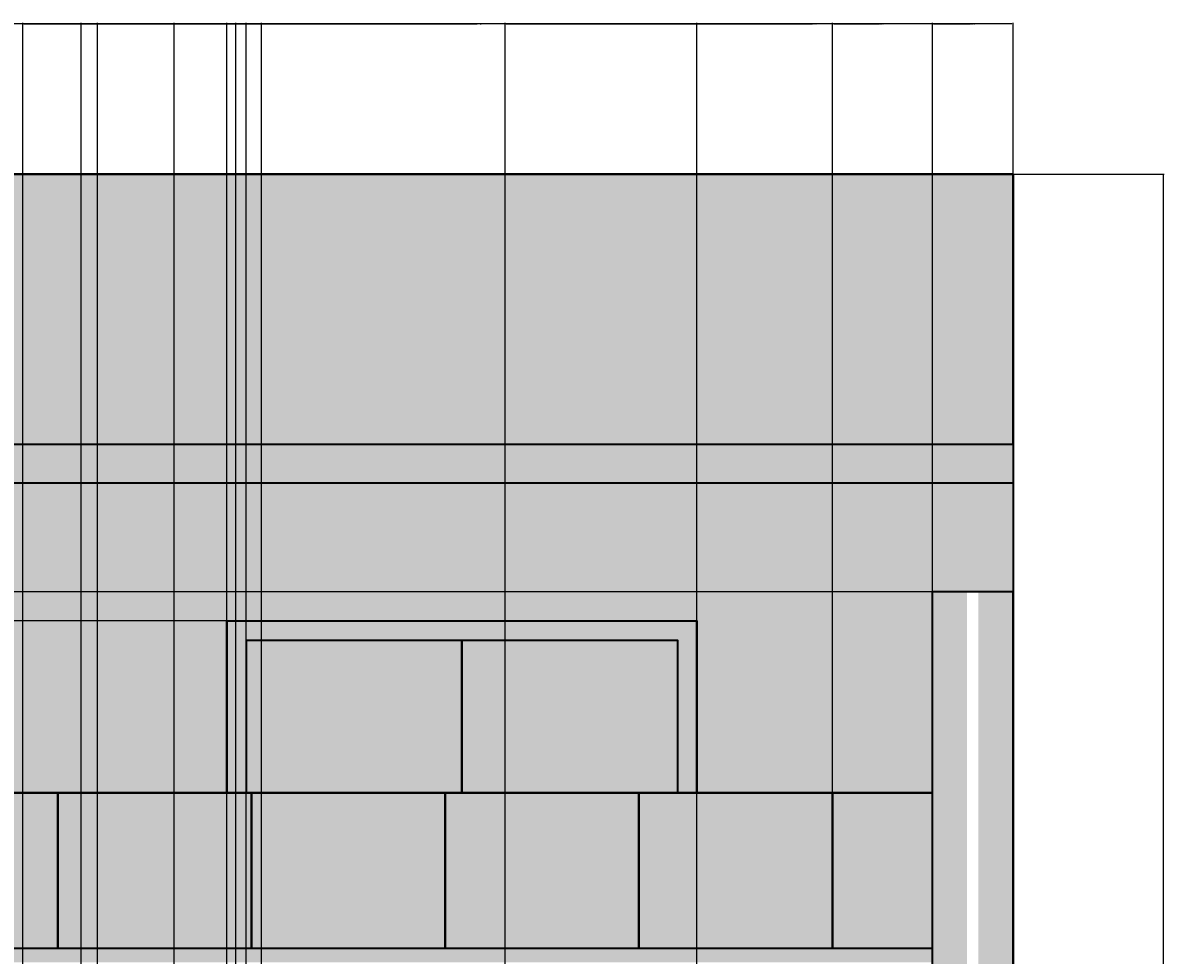
# Model space of a CAD drawing. Units: feet. Extents: x 2368 to 2738, y 1285 to 1782.
# Tile 6 of 6: x 2561 to 2738, y 1638 to 1782. Entities that reach past the tile are written whole.
import ezdxf

# ---------------------------------------------------------------- set-up
doc = ezdxf.new("R2010")
doc.units = ezdxf.units.FT
for name, color, linetype, lineweight in [('A-ANNO-DIMS', 2, 'Continuous', 18), ('A-ELEV', 7, 'Continuous', 35), ('A-ELEV-PATT', 252, 'Continuous', 13), ('A-GLAZ', 4, 'Continuous', 25)]:
    doc.layers.add(name, color=color, linetype=linetype, lineweight=lineweight)
doc.styles.get("Standard").update_dxf_attribs({"font": 'arial.ttf'})
doc.dimstyles.get("Standard").update_dxf_attribs({"dimtxt": 0.18, "dimasz": 0.18, "dimexe": 0.18, "dimexo": 0.0625, "dimgap": 0.09, "dimtad": 0, "dimtih": 1, "dimtoh": 1, "dimdec": 1, "dimzin": 0, "dimdsep": 46, "dimlunit": 3, "dimtxsty": 'Standard', "dimcen": 0.09, "dimadec": 0, "dimazin": 0, "dimtfac": 1, "dimtdec": 1, "dimtofl": 0, "dimtmove": 0, "dimatfit": 3, "dimfxl": 1, "dimtolj": 1, "dimtzin": 0, "dimarcsym": 0})

# ---------------------------------------------------------------- blocks, each defined once
blk = doc.blocks.new('*D1')
at = {"layer": 'A-ANNO-DIMS', "color": 0, "lineweight": -2, "transparency": 16777216}
for p, q in [((2391.54, 1662.92), (2391.54, 1782.11)), ((2391.72, 1781.93), (2552.46, 1781.93)), ((2713.98, 1781.93), (2553.25, 1781.93)), ((2714.16, 1758.74), (2714.16, 1782.11))]:
    blk.add_line(p, q, dxfattribs=at)
at = {"layer": 'A-ANNO-DIMS', "color": 0, "transparency": 16777216}
for points in [[(2391.72, 1781.96), (2391.72, 1781.9), (2391.54, 1781.93)], [(2713.98, 1781.96), (2713.98, 1781.9), (2714.16, 1781.93)]]:
    blk.add_solid(points, dxfattribs=at)
at = {"layer": 'Defpoints', "color": 0, "transparency": 16777216}
for p in [(2714.16, 1781.93), (2714.16, 1758.68), (2391.54, 1662.86)]:
    blk.add_point(p, dxfattribs=at)
at = {"layer": 'A-ANNO-DIMS', "color": 0, "transparency": 16777216, "insert": (2552.85, 1781.93), "char_height": 0.18, "attachment_point": 5}
blk.add_mtext('\\A1;322.6', dxfattribs=at)
blk = doc.blocks.new('*D2')
at = {"layer": 'A-ANNO-DIMS', "color": 0, "lineweight": -2, "transparency": 16777216}
for p, q in [((2714.23, 1758.68), (2737.59, 1758.68)), ((2737.41, 1758.5), (2737.41, 1533.95)), ((2737.41, 1309.04), (2737.41, 1533.58)), ((2714.23, 1308.86), (2737.59, 1308.86))]:
    blk.add_line(p, q, dxfattribs=at)
at = {"layer": 'A-ANNO-DIMS', "color": 0, "transparency": 16777216}
for points in [[(2737.38, 1758.5), (2737.44, 1758.5), (2737.41, 1758.68)], [(2737.38, 1309.04), (2737.44, 1309.04), (2737.41, 1308.86)]]:
    blk.add_solid(points, dxfattribs=at)
at = {"layer": 'Defpoints', "color": 0, "transparency": 16777216}
for p in [(2714.16, 1758.68), (2737.41, 1758.68), (2714.16, 1308.86)]:
    blk.add_point(p, dxfattribs=at)
at = {"layer": 'A-ANNO-DIMS', "color": 0, "transparency": 16777216, "insert": (2737.41, 1533.77), "char_height": 0.18, "attachment_point": 5}
blk.add_mtext('\\A1;449.8', dxfattribs=at)
blk = doc.blocks.new('*D33')
at = {"layer": 'A-ANNO-DIMS', "color": 0, "lineweight": -2, "transparency": 16777216}
for p, q in [((2592.41, 1461.2), (2592.41, 1782.11)), ((2592.59, 1781.93), (2593.76, 1781.93)), ((2595.23, 1781.93), (2594.06, 1781.93)), ((2595.41, 1458.2), (2595.41, 1782.11))]:
    blk.add_line(p, q, dxfattribs=at)
at = {"layer": 'A-ANNO-DIMS', "color": 0, "transparency": 16777216}
for points in [[(2592.59, 1781.96), (2592.59, 1781.9), (2592.41, 1781.93)], [(2595.23, 1781.96), (2595.23, 1781.9), (2595.41, 1781.93)]]:
    blk.add_solid(points, dxfattribs=at)
at = {"layer": 'Defpoints', "color": 0, "transparency": 16777216}
for p in [(2595.41, 1781.93), (2592.41, 1461.14), (2595.41, 1458.14)]:
    blk.add_point(p, dxfattribs=at)
at = {"layer": 'A-ANNO-DIMS', "color": 0, "transparency": 16777216, "insert": (2593.91, 1781.93), "char_height": 0.18, "attachment_point": 5}
blk.add_mtext('\\A1;3', dxfattribs=at)
blk = doc.blocks.new('*D34')
at = {"layer": 'A-ANNO-DIMS', "color": 0, "lineweight": -2, "transparency": 16777216}
for p, q in [((2560.8, 1466.16), (2560.8, 1782.11)), ((2560.98, 1781.93), (2597.75, 1781.93)), ((2635.31, 1781.93), (2598.54, 1781.93)), ((2635.49, 1466.16), (2635.49, 1782.11))]:
    blk.add_line(p, q, dxfattribs=at)
at = {"layer": 'A-ANNO-DIMS', "color": 0, "transparency": 16777216}
for points in [[(2560.98, 1781.96), (2560.98, 1781.9), (2560.8, 1781.93)], [(2635.31, 1781.96), (2635.31, 1781.9), (2635.49, 1781.93)]]:
    blk.add_solid(points, dxfattribs=at)
at = {"layer": 'Defpoints', "color": 0, "transparency": 16777216}
for p in [(2635.49, 1781.93), (2560.8, 1466.1), (2635.49, 1466.1)]:
    blk.add_point(p, dxfattribs=at)
at = {"layer": 'A-ANNO-DIMS', "color": 0, "transparency": 16777216, "insert": (2598.14, 1781.93), "char_height": 0.18, "attachment_point": 5}
blk.add_mtext('\\A1;74.69', dxfattribs=at)
blk = doc.blocks.new('*D35')
at = {"layer": 'A-ANNO-DIMS', "color": 0, "lineweight": -2, "transparency": 16777216}
for p, q in [((2635.49, 1466.16), (2635.49, 1782.11)), ((2635.67, 1781.93), (2668.18, 1781.93)), ((2701.48, 1781.93), (2668.97, 1781.93)), ((2701.66, 1466.16), (2701.66, 1782.11))]:
    blk.add_line(p, q, dxfattribs=at)
at = {"layer": 'A-ANNO-DIMS', "color": 0, "transparency": 16777216}
for points in [[(2635.67, 1781.96), (2635.67, 1781.9), (2635.49, 1781.93)], [(2701.48, 1781.96), (2701.48, 1781.9), (2701.66, 1781.93)]]:
    blk.add_solid(points, dxfattribs=at)
at = {"layer": 'Defpoints', "color": 0, "transparency": 16777216}
for p in [(2701.66, 1781.93), (2635.49, 1466.1), (2701.66, 1466.1)]:
    blk.add_point(p, dxfattribs=at)
at = {"layer": 'A-ANNO-DIMS', "color": 0, "transparency": 16777216, "insert": (2668.57, 1781.93), "char_height": 0.18, "attachment_point": 5}
blk.add_mtext('\\A1;66.17', dxfattribs=at)
blk = doc.blocks.new('*D39')
at = {"layer": 'A-ANNO-DIMS', "color": 0, "lineweight": -2, "transparency": 16777216}
for p, q in [((2701.6, 1662.86), (2368.11, 1662.86)), ((2368.29, 1662.68), (2368.29, 1651.02)), ((2368.29, 1638.99), (2368.29, 1650.65)), ((2701.6, 1638.81), (2368.11, 1638.81))]:
    blk.add_line(p, q, dxfattribs=at)
at = {"layer": 'A-ANNO-DIMS', "color": 0, "transparency": 16777216}
for points in [[(2368.26, 1662.68), (2368.32, 1662.68), (2368.29, 1662.86)], [(2368.26, 1638.99), (2368.32, 1638.99), (2368.29, 1638.81)]]:
    blk.add_solid(points, dxfattribs=at)
at = {"layer": 'Defpoints', "color": 0, "transparency": 16777216}
for p in [(2368.29, 1662.86), (2701.66, 1662.86), (2701.66, 1638.81)]:
    blk.add_point(p, dxfattribs=at)
at = {"layer": 'A-ANNO-DIMS', "color": 0, "transparency": 16777216, "insert": (2368.29, 1650.83), "char_height": 0.18, "attachment_point": 5}
blk.add_mtext('\\A1;24.042', dxfattribs=at)
blk = doc.blocks.new('*D40')
at = {"layer": 'A-ANNO-DIMS', "color": 0, "lineweight": -2, "transparency": 16777216}
for p, q in [((2701.6, 1693.98), (2368.11, 1693.98)), ((2368.29, 1693.8), (2368.29, 1678.6)), ((2368.29, 1663.04), (2368.29, 1678.24)), ((2701.6, 1662.86), (2368.11, 1662.86))]:
    blk.add_line(p, q, dxfattribs=at)
at = {"layer": 'A-ANNO-DIMS', "color": 0, "transparency": 16777216}
for points in [[(2368.26, 1693.8), (2368.32, 1693.8), (2368.29, 1693.98)], [(2368.26, 1663.04), (2368.32, 1663.04), (2368.29, 1662.86)]]:
    blk.add_solid(points, dxfattribs=at)
at = {"layer": 'Defpoints', "color": 0, "transparency": 16777216}
for p in [(2368.29, 1693.98), (2701.66, 1693.98), (2701.66, 1662.86)]:
    blk.add_point(p, dxfattribs=at)
at = {"layer": 'A-ANNO-DIMS', "color": 0, "transparency": 16777216, "insert": (2368.29, 1678.42), "char_height": 0.18, "attachment_point": 5}
blk.add_mtext('\\A1;31.13', dxfattribs=at)
blk = doc.blocks.new('*D54')
at = {"layer": 'A-ANNO-DIMS', "color": 0, "lineweight": -2, "transparency": 16777216}
for p, q in [((2560.78, 1609.97), (2560.78, 1782.11)), ((2560.96, 1781.93), (2564.98, 1781.93)), ((2569.66, 1781.93), (2565.63, 1781.93)), ((2569.84, 1609.97), (2569.84, 1782.11))]:
    blk.add_line(p, q, dxfattribs=at)
at = {"layer": 'A-ANNO-DIMS', "color": 0, "transparency": 16777216}
for points in [[(2560.96, 1781.96), (2560.96, 1781.9), (2560.78, 1781.93)], [(2569.66, 1781.96), (2569.66, 1781.9), (2569.84, 1781.93)]]:
    blk.add_solid(points, dxfattribs=at)
at = {"layer": 'Defpoints', "color": 0, "transparency": 16777216}
for p in [(2569.84, 1781.93), (2560.78, 1609.91), (2569.84, 1609.91)]:
    blk.add_point(p, dxfattribs=at)
at = {"layer": 'A-ANNO-DIMS', "color": 0, "transparency": 16777216, "insert": (2565.31, 1781.93), "char_height": 0.18, "attachment_point": 5}
blk.add_mtext('\\A1;9.06', dxfattribs=at)
blk = doc.blocks.new('*D55')
at = {"layer": 'A-ANNO-DIMS', "color": 0, "lineweight": -2, "transparency": 16777216}
for p, q in [((2569.84, 1609.97), (2569.84, 1782.11)), ((2570.02, 1781.93), (2576.72, 1781.93)), ((2584.06, 1781.93), (2577.35, 1781.93)), ((2584.24, 1609.97), (2584.24, 1782.11))]:
    blk.add_line(p, q, dxfattribs=at)
at = {"layer": 'A-ANNO-DIMS', "color": 0, "transparency": 16777216}
for points in [[(2570.02, 1781.96), (2570.02, 1781.9), (2569.84, 1781.93)], [(2584.06, 1781.96), (2584.06, 1781.9), (2584.24, 1781.93)]]:
    blk.add_solid(points, dxfattribs=at)
at = {"layer": 'Defpoints', "color": 0, "transparency": 16777216}
for p in [(2584.24, 1781.93), (2569.84, 1609.91), (2584.24, 1609.91)]:
    blk.add_point(p, dxfattribs=at)
at = {"layer": 'A-ANNO-DIMS', "color": 0, "transparency": 16777216, "insert": (2577.04, 1781.93), "char_height": 0.18, "attachment_point": 5}
blk.add_mtext('\\A1;14.4', dxfattribs=at)
blk = doc.blocks.new('*D56')
at = {"layer": 'A-ANNO-DIMS', "color": 0, "lineweight": -2, "transparency": 16777216}
for p, q in [((2593.78, 1609.97), (2593.78, 1782.11)), ((2593.96, 1781.93), (2595.62, 1781.93)), ((2597.6, 1781.93), (2595.93, 1781.93)), ((2597.78, 1609.97), (2597.78, 1782.11))]:
    blk.add_line(p, q, dxfattribs=at)
at = {"layer": 'A-ANNO-DIMS', "color": 0, "transparency": 16777216}
for points in [[(2593.96, 1781.96), (2593.96, 1781.9), (2593.78, 1781.93)], [(2597.6, 1781.96), (2597.6, 1781.9), (2597.78, 1781.93)]]:
    blk.add_solid(points, dxfattribs=at)
at = {"layer": 'Defpoints', "color": 0, "transparency": 16777216}
for p in [(2597.78, 1781.93), (2593.78, 1609.91), (2597.78, 1609.91)]:
    blk.add_point(p, dxfattribs=at)
at = {"layer": 'A-ANNO-DIMS', "color": 0, "transparency": 16777216, "insert": (2595.78, 1781.93), "char_height": 0.18, "attachment_point": 5}
blk.add_mtext('\\A1;4', dxfattribs=at)
blk = doc.blocks.new('*D57')
at = {"layer": 'A-ANNO-DIMS', "color": 0, "lineweight": -2, "transparency": 16777216}
for p, q in [((2569.84, 1609.97), (2569.84, 1782.11)), ((2570.02, 1781.93), (2570.71, 1781.93)), ((2572.19, 1781.93), (2571.5, 1781.93)), ((2572.37, 1609.97), (2572.37, 1782.11))]:
    blk.add_line(p, q, dxfattribs=at)
at = {"layer": 'A-ANNO-DIMS', "color": 0, "transparency": 16777216}
for points in [[(2570.02, 1781.96), (2570.02, 1781.9), (2569.84, 1781.93)], [(2572.19, 1781.96), (2572.19, 1781.9), (2572.37, 1781.93)]]:
    blk.add_solid(points, dxfattribs=at)
at = {"layer": 'Defpoints', "color": 0, "transparency": 16777216}
for p in [(2572.37, 1781.93), (2569.84, 1609.91), (2572.37, 1609.91)]:
    blk.add_point(p, dxfattribs=at)
at = {"layer": 'A-ANNO-DIMS', "color": 0, "transparency": 16777216, "insert": (2571.11, 1781.93), "char_height": 0.18, "attachment_point": 5}
blk.add_mtext('\\A1;2.539', dxfattribs=at)
blk = doc.blocks.new('*D58')
at = {"layer": 'A-ANNO-DIMS', "color": 0, "lineweight": -2, "transparency": 16777216}
for p, q in [((2597.78, 1600.54), (2597.78, 1782.11)), ((2597.96, 1781.93), (2631.09, 1781.93)), ((2665.02, 1781.93), (2631.88, 1781.93)), ((2665.2, 1600.54), (2665.2, 1782.11))]:
    blk.add_line(p, q, dxfattribs=at)
at = {"layer": 'A-ANNO-DIMS', "color": 0, "transparency": 16777216}
for points in [[(2597.96, 1781.96), (2597.96, 1781.9), (2597.78, 1781.93)], [(2665.02, 1781.96), (2665.02, 1781.9), (2665.2, 1781.93)]]:
    blk.add_solid(points, dxfattribs=at)
at = {"layer": 'Defpoints', "color": 0, "transparency": 16777216}
for p in [(2665.2, 1781.93), (2597.78, 1600.48), (2665.2, 1600.48)]:
    blk.add_point(p, dxfattribs=at)
at = {"layer": 'A-ANNO-DIMS', "color": 0, "transparency": 16777216, "insert": (2631.49, 1781.93), "char_height": 0.18, "attachment_point": 5}
blk.add_mtext('\\A1;67.42', dxfattribs=at)
blk = doc.blocks.new('*D59')
at = {"layer": 'A-ANNO-DIMS', "color": 0, "lineweight": -2, "transparency": 16777216}
for p, q in [((2665.2, 1600.54), (2665.2, 1782.11)), ((2665.38, 1781.93), (2683.03, 1781.93)), ((2701.48, 1781.93), (2683.82, 1781.93)), ((2701.66, 1609.97), (2701.66, 1782.11))]:
    blk.add_line(p, q, dxfattribs=at)
at = {"layer": 'A-ANNO-DIMS', "color": 0, "transparency": 16777216}
for points in [[(2665.38, 1781.96), (2665.38, 1781.9), (2665.2, 1781.93)], [(2701.48, 1781.96), (2701.48, 1781.9), (2701.66, 1781.93)]]:
    blk.add_solid(points, dxfattribs=at)
at = {"layer": 'Defpoints', "color": 0, "transparency": 16777216}
for p in [(2701.66, 1781.93), (2701.66, 1609.91), (2665.2, 1600.48)]:
    blk.add_point(p, dxfattribs=at)
at = {"layer": 'A-ANNO-DIMS', "color": 0, "transparency": 16777216, "insert": (2683.43, 1781.93), "char_height": 0.18, "attachment_point": 5}
blk.add_mtext('\\A1;36.46', dxfattribs=at)
blk = doc.blocks.new('*D65')
at = {"layer": 'A-ANNO-DIMS', "color": 0, "lineweight": -2, "transparency": 16777216}
for p, q in [((2686.2, 1662.92), (2686.2, 1782.11)), ((2686.38, 1781.93), (2693.47, 1781.93)), ((2701.48, 1781.93), (2694.38, 1781.93)), ((2701.66, 1662.92), (2701.66, 1782.11))]:
    blk.add_line(p, q, dxfattribs=at)
at = {"layer": 'A-ANNO-DIMS', "color": 0, "transparency": 16777216}
for points in [[(2686.38, 1781.96), (2686.38, 1781.9), (2686.2, 1781.93)], [(2701.48, 1781.96), (2701.48, 1781.9), (2701.66, 1781.93)]]:
    blk.add_solid(points, dxfattribs=at)
at = {"layer": 'Defpoints', "color": 0, "transparency": 16777216}
for p in [(2701.66, 1781.93), (2686.2, 1662.86), (2701.66, 1662.86)]:
    blk.add_point(p, dxfattribs=at)
at = {"layer": 'A-ANNO-DIMS', "color": 0, "transparency": 16777216, "insert": (2693.93, 1781.93), "char_height": 0.18, "attachment_point": 5}
blk.add_mtext('\\A1;15.464', dxfattribs=at)
blk = doc.blocks.new('*D69')
at = {"layer": 'A-ANNO-DIMS', "color": 0, "lineweight": -2, "transparency": 16777216}
for p, q in [((2519.62, 1716.92), (2519.62, 1782.11)), ((2519.8, 1781.93), (2555.62, 1781.93)), ((2592.23, 1781.93), (2556.41, 1781.93)), ((2592.41, 1689.56), (2592.41, 1782.11))]:
    blk.add_line(p, q, dxfattribs=at)
at = {"layer": 'A-ANNO-DIMS', "color": 0, "transparency": 16777216}
for points in [[(2519.8, 1781.96), (2519.8, 1781.9), (2519.62, 1781.93)], [(2592.23, 1781.96), (2592.23, 1781.9), (2592.41, 1781.93)]]:
    blk.add_solid(points, dxfattribs=at)
at = {"layer": 'Defpoints', "color": 0, "transparency": 16777216}
for p in [(2592.41, 1781.93), (2519.62, 1716.86), (2592.41, 1689.49)]:
    blk.add_point(p, dxfattribs=at)
at = {"layer": 'A-ANNO-DIMS', "color": 0, "transparency": 16777216, "insert": (2556.02, 1781.93), "char_height": 0.18, "attachment_point": 5}
blk.add_mtext('\\A1;72.79', dxfattribs=at)
blk = doc.blocks.new('*D70')
at = {"layer": 'A-ANNO-DIMS', "color": 0, "lineweight": -2, "transparency": 16777216}
for p, q in [((2592.41, 1689.56), (2592.41, 1782.11)), ((2592.59, 1781.93), (2628.41, 1781.93)), ((2665.02, 1781.93), (2629.2, 1781.93)), ((2665.2, 1689.56), (2665.2, 1782.11))]:
    blk.add_line(p, q, dxfattribs=at)
at = {"layer": 'A-ANNO-DIMS', "color": 0, "transparency": 16777216}
for points in [[(2592.59, 1781.96), (2592.59, 1781.9), (2592.41, 1781.93)], [(2665.02, 1781.96), (2665.02, 1781.9), (2665.2, 1781.93)]]:
    blk.add_solid(points, dxfattribs=at)
at = {"layer": 'Defpoints', "color": 0, "transparency": 16777216}
for p in [(2665.2, 1781.93), (2592.41, 1689.49), (2665.2, 1689.49)]:
    blk.add_point(p, dxfattribs=at)
at = {"layer": 'A-ANNO-DIMS', "color": 0, "transparency": 16777216, "insert": (2628.8, 1781.93), "char_height": 0.18, "attachment_point": 5}
blk.add_mtext('\\A1;72.78', dxfattribs=at)
blk = doc.blocks.new('*D71')
at = {"layer": 'A-ANNO-DIMS', "color": 0, "lineweight": -2, "transparency": 16777216}
for p, q in [((2592.35, 1689.49), (2368.11, 1689.49)), ((2368.29, 1689.31), (2368.29, 1676.36)), ((2368.29, 1663.04), (2368.29, 1675.99)), ((2592.35, 1662.86), (2368.11, 1662.86))]:
    blk.add_line(p, q, dxfattribs=at)
at = {"layer": 'A-ANNO-DIMS', "color": 0, "transparency": 16777216}
for points in [[(2368.26, 1689.31), (2368.32, 1689.31), (2368.29, 1689.49)], [(2368.26, 1663.04), (2368.32, 1663.04), (2368.29, 1662.86)]]:
    blk.add_solid(points, dxfattribs=at)
at = {"layer": 'Defpoints', "color": 0, "transparency": 16777216}
for p in [(2368.29, 1689.49), (2592.41, 1689.49), (2592.41, 1662.86)]:
    blk.add_point(p, dxfattribs=at)
at = {"layer": 'A-ANNO-DIMS', "color": 0, "transparency": 16777216, "insert": (2368.29, 1676.17), "char_height": 0.18, "attachment_point": 5}
blk.add_mtext('\\A1;26.64', dxfattribs=at)
blk = doc.blocks.new('*D72')
at = {"layer": 'A-ANNO-DIMS', "color": 0, "lineweight": -2, "transparency": 16777216}
for p, q in [((2592.41, 1689.56), (2592.41, 1782.11)), ((2592.59, 1781.93), (2593.76, 1781.93)), ((2595.23, 1781.93), (2594.06, 1781.93)), ((2595.41, 1686.56), (2595.41, 1782.11))]:
    blk.add_line(p, q, dxfattribs=at)
at = {"layer": 'A-ANNO-DIMS', "color": 0, "transparency": 16777216}
for points in [[(2592.59, 1781.96), (2592.59, 1781.9), (2592.41, 1781.93)], [(2595.23, 1781.96), (2595.23, 1781.9), (2595.41, 1781.93)]]:
    blk.add_solid(points, dxfattribs=at)
at = {"layer": 'Defpoints', "color": 0, "transparency": 16777216}
for p in [(2595.41, 1781.93), (2592.41, 1689.49), (2595.41, 1686.49)]:
    blk.add_point(p, dxfattribs=at)
at = {"layer": 'A-ANNO-DIMS', "color": 0, "transparency": 16777216, "insert": (2593.91, 1781.93), "char_height": 0.18, "attachment_point": 5}
blk.add_mtext('\\A1;3', dxfattribs=at)
blk = doc.blocks.new('*D73')
at = {"layer": 'A-ANNO-DIMS', "color": 0, "lineweight": -2, "transparency": 16777216}
for p, q in [((2701.66, 1694.05), (2701.66, 1782.11)), ((2701.84, 1781.93), (2707.46, 1781.93)), ((2713.98, 1781.93), (2708.37, 1781.93)), ((2714.16, 1694.05), (2714.16, 1782.11))]:
    blk.add_line(p, q, dxfattribs=at)
at = {"layer": 'A-ANNO-DIMS', "color": 0, "transparency": 16777216}
for points in [[(2701.84, 1781.96), (2701.84, 1781.9), (2701.66, 1781.93)], [(2713.98, 1781.96), (2713.98, 1781.9), (2714.16, 1781.93)]]:
    blk.add_solid(points, dxfattribs=at)
at = {"layer": 'Defpoints', "color": 0, "transparency": 16777216}
for p in [(2714.16, 1781.93), (2701.66, 1693.98), (2714.16, 1693.98)]:
    blk.add_point(p, dxfattribs=at)
at = {"layer": 'A-ANNO-DIMS', "color": 0, "transparency": 16777216, "insert": (2707.91, 1781.93), "char_height": 0.18, "attachment_point": 5}
blk.add_mtext('\\A1;12.503', dxfattribs=at)

msp = doc.modelspace()

# ---------------------------------------------------------------- hatches: boundary and pattern name
at = {"layer": 'A-ELEV-PATT'}
h = msp.add_hatch(color=256, dxfattribs=at)
h.set_gradient(color1=(192, 192, 192), color2=(192, 192, 192), tint=1)
h.paths.add_polyline_path([(2714.1625, 1758.6751), (2519.621, 1758.6751), (2519.621, 1716.8552), (2714.1625, 1716.8552)])
h.paths.add_polyline_path([(2701.6591, 1693.9847), (2714.1625, 1693.9847), (2714.1625, 1710.8552), (2519.621, 1710.8552), (2519.621, 1662.8552), (2592.4132, 1662.8552), (2592.4132, 1689.493), (2665.1962, 1689.493), (2665.1962, 1662.8552), (2701.6591, 1662.8552)])
h.paths.add_polyline_path([(2701.6591, 1609.9058), (2597.776, 1609.9058), (2597.776, 1600.4784), (2665.1962, 1600.4784), (2665.1962, 1596.3371), (2665.1962, 1522.6314), (2701.6591, 1522.6314)])
h.paths.add_polyline_path([(2463.0324, 1598.097), (2536.677, 1598.097), (2536.677, 1519.7115), (2560.74, 1519.7115), (2560.5754, 1609.9058), (2542.3749, 1609.9058), (2441.2488, 1609.9058), (2441.2488, 1519.7115), (2463.0324, 1519.7115)])
h.paths.add_polyline_path([(2506.1956, 1662.8552), (2391.5414, 1662.8552), (2391.5414, 1644.4206), (2438.815, 1644.4206, -0.34592239), (2445.9507, 1638.8128), (2506.1956, 1638.8128)])
h.paths.add_polyline_path([(2410.9473, 1609.9058, -0.04175491), (2411.9608, 1614.8552), (2391.5414, 1614.8552), (2391.5414, 1488.8552), (2410.9473, 1488.8552)])
h.paths.add_polyline_path([(2426.5897, 1605.0962, 1), (2422.7862, 1605.0962), (2422.7862, 1509.5049, 1), (2426.5897, 1509.5049)])
h.paths.add_polyline_path([(2463.0324, 1460.097), (2536.677, 1460.097), (2536.677, 1350.8552), (2543.4468, 1350.8552), (2543.4468, 1482.8552), (2391.5414, 1482.8552), (2391.5414, 1350.8552), (2463.0324, 1350.8552)])
h.paths.add_polyline_path([(2436.8485, 1456.084), (2436.8485, 1379.669), (2399.9065, 1379.669), (2399.9065, 1456.084)], flags=16)
h.paths.add_polyline_path([(2434.8485, 1454.084), (2434.8485, 1381.669), (2401.9065, 1381.669), (2401.9065, 1454.084)], flags=0)
h.paths.add_polyline_path([(2714.1625, 1350.8552), (2391.5414, 1350.8552), (2391.5414, 1320.8552), (2714.1625, 1320.8552)])
h.paths.add_polyline_path([(2714.1625, 1320.8552), (2391.5414, 1320.8552), (2391.5414, 1308.8552), (2714.1625, 1308.8552)])
h = msp.add_hatch(color=256, dxfattribs=at)
h.set_gradient(color1=(128, 128, 128), color2=(128, 128, 128), tint=1)
h.paths.add_polyline_path([(2519.621, 1716.8552), (2409.5414, 1716.8552), (2409.5414, 1662.8552), (2415.5414, 1662.8552), (2415.5414, 1710.8552), (2519.621, 1710.8552)])
h.paths.add_polyline_path([(2714.1625, 1716.8552), (2519.621, 1716.8552), (2519.621, 1710.8552), (2714.1625, 1710.8552)])
h.paths.add_polyline_path([(2701.6591, 1638.8128), (2445.9507, 1638.8128, -0.0752442), (2446.1448, 1636.6235), (2542.3749, 1636.6235), (2542.776, 1636.6235), (2701.6591, 1636.6235)])
h = msp.add_hatch(color=256, dxfattribs=at)
h.set_gradient(color1=(255, 255, 255), tint=1)
h.paths.add_polyline_path([(2714.1625, 1693.9847), (2708.7975, 1693.9847), (2708.7975, 1466.101), (2714.1625, 1466.101)])
h.paths.add_polyline_path([(2707.0241, 1693.9847), (2701.6591, 1693.9847), (2701.6591, 1466.101), (2707.0241, 1466.101)])
h = msp.add_hatch(color=256, dxfattribs=at)
h.set_gradient(color1=(255, 255, 255), tint=1)
h.paths.add_polyline_path([(2595.4132, 1686.493), (2662.1962, 1686.493), (2662.1962, 1662.8552), (2665.1962, 1662.8552), (2665.1962, 1689.493), (2592.4132, 1689.493), (2592.4132, 1662.8552), (2595.4132, 1662.8552)])
h.paths.add_polyline_path([(2665.1962, 1600.4784), (2597.776, 1600.4784), (2597.776, 1597.4784), (2662.1962, 1597.4784), (2662.1962, 1510.3225), (2597.776, 1510.3225), (2597.776, 1507.3225), (2665.1962, 1507.3225)])
h.paths.add_polyline_path([(2665.1962, 1461.1396), (2592.4132, 1461.1396), (2592.4132, 1367.9838), (2665.1962, 1367.9838)])
h.paths.add_polyline_path([(2662.1962, 1458.1396), (2662.1962, 1370.9838), (2595.4132, 1370.9838), (2595.4132, 1458.1396)], flags=16)
h.paths.add_polyline_path([(2593.776, 1609.9058), (2584.2358, 1609.9058), (2584.2358, 1488.8552), (2593.776, 1488.8552)])
h.paths.add_polyline_path([(2597.776, 1609.9058), (2595.4517, 1609.9058), (2595.4517, 1488.8552), (2597.776, 1488.8552)])
h.paths.add_polyline_path([(2569.8357, 1609.9058), (2560.5754, 1609.9058), (2560.74, 1519.7115), (2560.7407, 1519.7115), (2560.7407, 1519.3328), (2560.7963, 1488.8552), (2569.8357, 1488.8552)])
h.paths.add_polyline_path([(2572.6807, 1609.9058), (2571.6967, 1609.9058), (2571.6967, 1488.8552), (2572.6807, 1488.8552)])
h.paths.add_polyline_path([(2575.8428, 1609.9058), (2574.5416, 1609.9058), (2574.5416, 1488.8552), (2575.8428, 1488.8552)])
h.paths.add_polyline_path([(2579.0308, 1609.9058), (2577.7037, 1609.9058), (2577.7037, 1488.8552), (2579.0308, 1488.8552)])
h.paths.add_polyline_path([(2582.3749, 1609.9058), (2580.8918, 1609.9058), (2580.8918, 1488.8552), (2582.3749, 1488.8552)])
h = msp.add_hatch(color=256, dxfattribs=at)
h.set_gradient(color1=(0, 255, 255), color2=(0, 255, 255), tint=1)
h.paths.add_polyline_path([(2418.2281, 1454.084), (2401.9065, 1454.084), (2401.9065, 1381.669), (2418.2281, 1381.669)])
h.paths.add_polyline_path([(2434.8485, 1454.084), (2418.5148, 1454.084), (2418.5148, 1381.669), (2434.8485, 1381.669)])
h.paths.add_polyline_path([(2662.1962, 1458.1396), (2595.4132, 1458.1396), (2595.4132, 1414.5617), (2662.1962, 1414.5617)])
h.paths.add_polyline_path([(2662.1962, 1414.5617), (2628.8047, 1414.5617), (2628.8047, 1370.9838), (2662.1962, 1370.9838)])
h.paths.add_polyline_path([(2628.8047, 1414.5617), (2595.4132, 1414.5617), (2595.4132, 1370.9838), (2628.8047, 1370.9838)])
h.paths.add_polyline_path([(2662.1962, 1597.4784), (2628.8047, 1597.4784), (2628.8047, 1553.9004), (2662.1962, 1553.9004)])
h.paths.add_polyline_path([(2628.8047, 1597.4784), (2597.776, 1597.4784), (2597.776, 1553.9004), (2628.8047, 1553.9004)])
h.paths.add_polyline_path([(2628.8047, 1553.9004), (2597.776, 1553.9004), (2597.776, 1522.6314), (2628.8047, 1522.6314)])
h.paths.add_polyline_path([(2662.1962, 1553.9004), (2628.8047, 1553.9004), (2628.8047, 1522.6314), (2662.1962, 1522.6314)])
h.paths.add_polyline_path([(2662.1962, 1686.493), (2628.8047, 1686.493), (2628.8047, 1662.8552), (2662.1962, 1662.8552)])
h.paths.add_polyline_path([(2628.8047, 1686.493), (2595.4132, 1686.493), (2595.4132, 1662.8552), (2628.8047, 1662.8552)])
h = msp.add_hatch(color=256, dxfattribs=at)
h.set_gradient(color1=(153, 185, 219), color2=(153, 185, 219), tint=1)
h.paths.add_polyline_path([(2536.1956, 1662.8552), (2506.1956, 1662.8552), (2506.1956, 1638.8128), (2536.1956, 1638.8128)])
h.paths.add_polyline_path([(2566.1956, 1662.8552), (2536.1956, 1662.8552), (2536.1956, 1638.8128), (2566.1956, 1638.8128)])
h.paths.add_polyline_path([(2596.1956, 1662.8552), (2566.1956, 1662.8552), (2566.1956, 1638.8128), (2596.1956, 1638.8128)])
h.paths.add_polyline_path([(2626.1956, 1662.8552), (2596.1956, 1662.8552), (2596.1956, 1638.8128), (2626.1956, 1638.8128)])
h.paths.add_polyline_path([(2656.1956, 1662.8552), (2626.1956, 1662.8552), (2626.1956, 1638.8128), (2656.1956, 1638.8128)])
h.paths.add_polyline_path([(2686.1956, 1662.8552), (2656.1956, 1662.8552), (2656.1956, 1638.8128), (2686.1956, 1638.8128)])
h.paths.add_polyline_path([(2701.6591, 1662.8552), (2686.1956, 1662.8552), (2686.1956, 1638.8128), (2701.6591, 1638.8128)])

# ---------------------------------------------------------------- linework, layer by layer
at = {"layer": 'A-ELEV'}
for p, q in [((2519.621, 1758.6751), (2714.1625, 1758.6751)), ((2714.1625, 1758.6751), (2519.621, 1758.6751)), ((2714.1625, 1716.8552), (2714.1625, 1758.6751)), ((2714.1625, 1716.8552), (2714.1625, 1758.6751)), ((2714.1625, 1758.6751), (2714.1625, 1693.9847)), ((2409.5414, 1716.8552), (2714.1625, 1716.8552)), ((2519.621, 1716.8552), (2714.1625, 1716.8552)), ((2415.5414, 1710.8552), (2714.1625, 1710.8552)), ((2519.662, 1710.8552), (2714.1625, 1710.8552)), ((2714.1625, 1693.9847), (2701.6591, 1693.9847)), ((2701.6591, 1693.9847), (2701.6591, 1466.101)), ((2714.1625, 1466.101), (2714.1625, 1693.9847)), ((2592.4132, 1689.493), (2592.4132, 1662.8552)), ((2665.1962, 1662.8552), (2665.1962, 1689.493)), ((2595.4132, 1662.8552), (2595.4132, 1686.493)), ((2628.8047, 1686.493), (2628.8047, 1662.8552)), ((2662.1962, 1686.493), (2662.1962, 1662.8552)), ((2391.5414, 1662.8552), (2701.6591, 1662.8552)), ((2701.6591, 1662.8552), (2391.5414, 1662.8552)), ((2566.1956, 1662.8552), (2566.1956, 1638.8128)), ((2566.1956, 1638.8128), (2566.1956, 1662.8552)), ((2596.1956, 1662.8552), (2596.1956, 1638.8128)), ((2596.1956, 1638.8128), (2596.1956, 1662.8552)), ((2626.1956, 1662.8552), (2626.1956, 1638.8128)), ((2626.1956, 1638.8128), (2626.1956, 1662.8552)), ((2656.1956, 1662.8552), (2656.1956, 1638.8128)), ((2656.1956, 1638.8128), (2656.1956, 1662.8552)), ((2686.1956, 1662.8552), (2686.1956, 1638.8128)), ((2686.1956, 1638.8128), (2686.1956, 1662.8552)), ((2445.9507, 1638.8128), (2701.6591, 1638.8128)), ((2445.9507, 1638.8128), (2701.6591, 1638.8128))]:
    msp.add_line(p, q, dxfattribs=at)
for points in [[(2714.1625, 1716.8552), (2714.1625, 1308.8552)], [(2592.4132, 1662.8552), (2592.4132, 1689.493), (2665.1962, 1689.493), (2665.1962, 1662.8552)], [(2595.4132, 1662.8552), (2595.4132, 1686.493), (2662.1962, 1686.493), (2662.1962, 1662.8552)]]:
    msp.add_lwpolyline(points, dxfattribs=at)
for points in [[(2714.1625, 1693.9847), (2701.6591, 1693.9847), (2701.6591, 1466.101), (2714.1625, 1466.101)], [(2628.8047, 1686.493), (2628.8047, 1686.493), (2628.8047, 1662.8552), (2628.8047, 1662.8552)]]:
    msp.add_lwpolyline(points, close=True, dxfattribs=at)
at = {"layer": 'A-GLAZ'}
for p, q in [((2665.1962, 1689.493), (2592.4132, 1689.493)), ((2595.4132, 1686.493), (2662.1962, 1686.493))]:
    msp.add_line(p, q, dxfattribs=at)

# ---------------------------------------------------------------- dimensions: what is measured, and where the dimension line sits
at = {"layer": 'A-ANNO-DIMS'}
for base, p1, p2, override, picture, middle in [((2714.1625, 1781.9251), (2391.5414, 1662.8552), (2714.1625, 1758.6751), {"dimdec": 1, "dimlfac": 1, "dimrnd": 0, "dimzin": 0, "dimdsep": 46, "dimlunit": 2}, '*D1', (2552.8519, 1781.9251)), ((2592.4132, 1781.9251), (2519.621, 1716.8552), (2592.4132, 1689.493), {"dimdec": 2, "dimlfac": 1, "dimrnd": 0, "dimzin": 0, "dimdsep": 46, "dimlunit": 2}, '*D69', (2556.0171, 1781.9251)), ((2569.8357, 1781.9251), (2560.776, 1609.9058), (2569.8357, 1609.9058), {"dimdec": 2, "dimlfac": 1, "dimrnd": 0, "dimzin": 0, "dimdsep": 46, "dimlunit": 2}, '*D54', (2565.3059, 1781.9251)), ((2635.4878, 1781.9251), (2560.7963, 1466.101), (2635.4878, 1466.101), {"dimdec": 2, "dimlfac": 1, "dimrnd": 0, "dimzin": 0, "dimdsep": 46, "dimlunit": 2}, '*D34', (2598.1421, 1781.9251)), ((2584.2358, 1781.9251), (2569.8357, 1609.9058), (2584.2358, 1609.9058), {"dimdec": 1, "dimlfac": 1, "dimrnd": 0, "dimzin": 0, "dimdsep": 46, "dimlunit": 2}, '*D55', (2577.0358, 1781.9251)), ((2572.3749, 1781.9251), (2569.8357, 1609.9058), (2572.3749, 1609.9058), {"dimdec": 3, "dimlfac": 1, "dimrnd": 0, "dimzin": 0, "dimdsep": 46, "dimlunit": 2}, '*D57', (2571.1053, 1781.9251)), ((2595.4132, 1781.9251), (2592.4132, 1461.1396), (2595.4132, 1458.1396), {"dimdec": 0, "dimlfac": 1, "dimrnd": 0, "dimzin": 0, "dimdsep": 46, "dimlunit": 2}, '*D33', (2593.9132, 1781.9251)), ((2665.1962, 1781.9251), (2592.4132, 1689.493), (2665.1962, 1689.493), {"dimdec": 2, "dimlfac": 1, "dimrnd": 0, "dimzin": 0, "dimdsep": 46, "dimlunit": 2}, '*D70', (2628.8047, 1781.9251)), ((2595.4132, 1781.9251), (2592.4132, 1689.493), (2595.4132, 1686.493), {"dimdec": 0, "dimlfac": 1, "dimrnd": 0, "dimzin": 0, "dimdsep": 46, "dimlunit": 2}, '*D72', (2593.9132, 1781.9251)), ((2597.776, 1781.9251), (2593.776, 1609.9058), (2597.776, 1609.9058), {"dimdec": 0, "dimlfac": 1, "dimrnd": 0, "dimzin": 0, "dimdsep": 46, "dimlunit": 2}, '*D56', (2595.776, 1781.9251)), ((2665.1962, 1781.9251), (2597.776, 1600.4784), (2665.1962, 1600.4784), {"dimdec": 2, "dimlfac": 1, "dimrnd": 0, "dimzin": 0, "dimdsep": 46, "dimlunit": 2}, '*D58', (2631.4861, 1781.9251)), ((2701.6591, 1781.9251), (2635.4878, 1466.101), (2701.6591, 1466.101), {"dimdec": 2, "dimlfac": 1, "dimrnd": 0, "dimzin": 0, "dimdsep": 46, "dimlunit": 2}, '*D35', (2668.5735, 1781.9251)), ((2701.6591, 1781.9251), (2665.1962, 1600.4784), (2701.6591, 1609.9058), {"dimdec": 2, "dimlfac": 1, "dimrnd": 0, "dimzin": 0, "dimdsep": 46, "dimlunit": 2}, '*D59', (2683.4277, 1781.9251)), ((2701.65914, 1781.9251), (2686.19556, 1662.85522), (2701.65914, 1662.85522), {"dimdec": 3, "dimlfac": 1, "dimrnd": 0, "dimzin": 0, "dimdsep": 46, "dimlunit": 2}, '*D65', (2693.92735, 1781.9251)), ((2714.1625, 1781.9251), (2701.6591, 1693.9847), (2714.1625, 1693.9847), {"dimdec": 3, "dimlfac": 1, "dimrnd": 0, "dimzin": 0, "dimdsep": 46, "dimlunit": 2}, '*D73', (2707.9108, 1781.9251))]:
    dim = msp.add_linear_dim(base=base, p1=p1, p2=p2, dimstyle='Standard', override=override, dxfattribs=at)
    dim.commit()
    dim.dimension.update_dxf_attribs({"geometry": picture, "text_midpoint": middle})
for base, p1, p2, override, picture, middle in [((2737.4125, 1758.6751), (2714.1625, 1308.8552), (2714.1625, 1758.6751), {"dimdec": 1, "dimlfac": 1, "dimrnd": 0, "dimzin": 0, "dimdsep": 46, "dimlunit": 2}, '*D2', (2737.4125, 1533.7652)), ((2368.2914, 1693.9847), (2701.6591, 1662.8552), (2701.6591, 1693.9847), {"dimdec": 2, "dimlfac": 1, "dimrnd": 0, "dimzin": 0, "dimdsep": 46, "dimlunit": 2}, '*D40', (2368.2914, 1678.42)), ((2368.2914, 1689.493), (2592.4132, 1662.8552), (2592.4132, 1689.493), {"dimdec": 2, "dimlfac": 1, "dimrnd": 0, "dimzin": 0, "dimdsep": 46, "dimlunit": 2}, '*D71', (2368.2914, 1676.1741)), ((2368.2914, 1662.8552), (2701.6591, 1638.8128), (2701.6591, 1662.8552), {"dimdec": 3, "dimlfac": 1, "dimrnd": 0, "dimzin": 0, "dimdsep": 46, "dimlunit": 2}, '*D39', (2368.2914, 1650.834))]:
    dim = msp.add_linear_dim(base=base, p1=p1, p2=p2, angle=90, dimstyle='Standard', override=override, dxfattribs=at)
    dim.commit()
    dim.dimension.update_dxf_attribs({"geometry": picture, "text_midpoint": middle})

doc.saveas('drawing.dxf')
